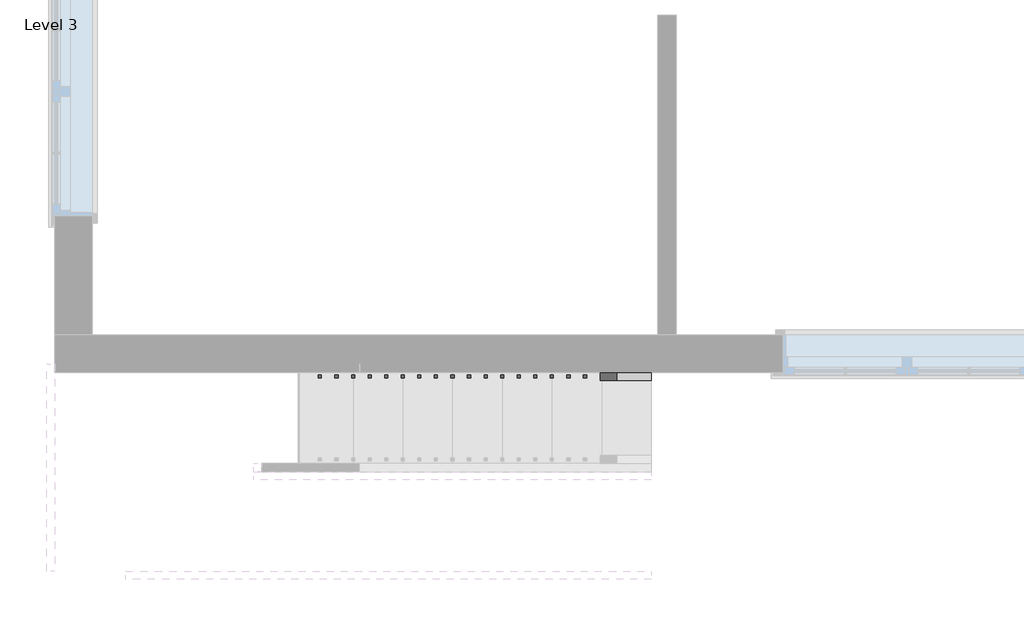
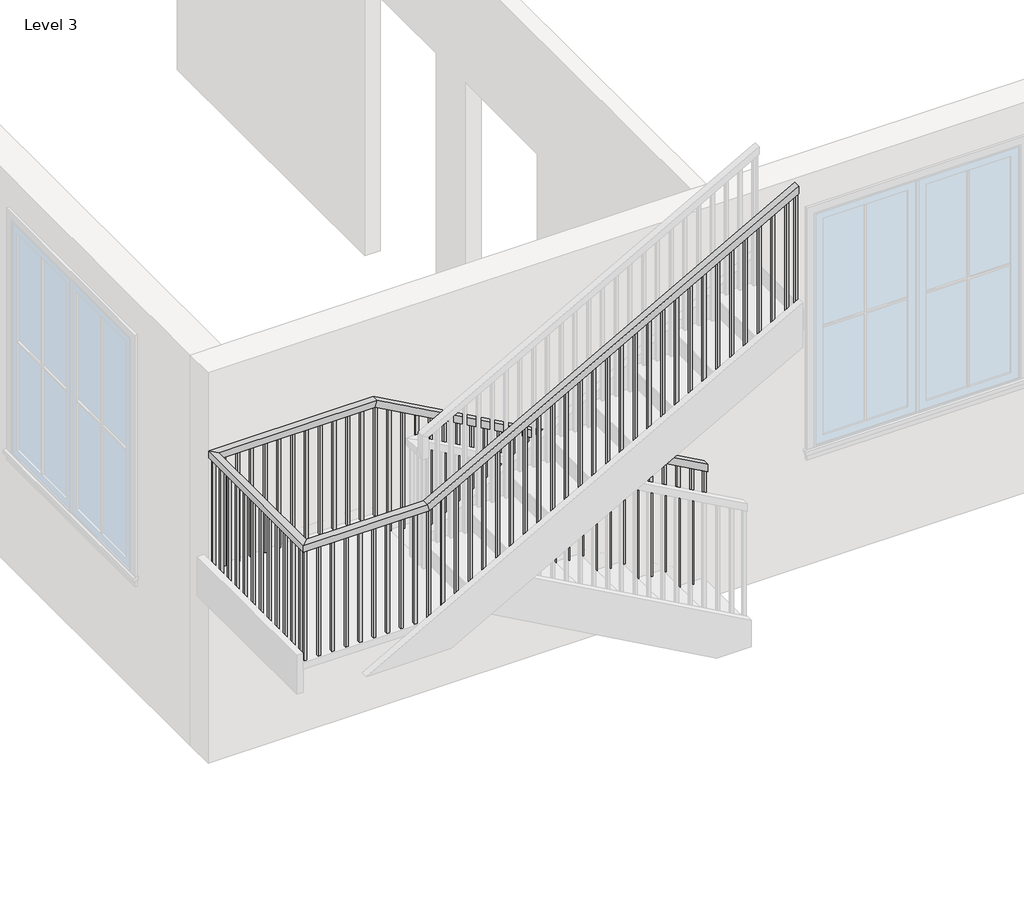
# One storey, part 2 of 3: 1 railing.
"""IFC4 building model written with IfcOpenShell, lengths in millimetres."""

from ifc_helpers import new_model, si_unit, frame, origin, place, context, project, spatial, polyline, outline, extrude, faceted_brep, element, save

model = new_model("IFC4")

# Units and contexts
model_context = context("Model", 3, world=origin())
ifc_project = project(units=[si_unit("LENGTHUNIT", "METRE", prefix="MILLI")], contexts=[model_context])

# Site, building, storey
site = spatial("IfcSite", under=ifc_project)
building = spatial("IfcBuilding", under=site)
storey = spatial("IfcBuildingStorey", under=building, Name="Level 3", Elevation=3200.4)

# Railing
placement = place(None, origin())
element("IfcRailing", 1, ObjectType="Handrail - Rectangular", at=placement, inside=storey, context=model_context, shape_type="SolidModel", body=[
    faceted_brep([(-1805.9198569, -5357.1933037, 4284.1333333), (-1805.9198569, -5357.1933037, 4226.020221), (-1805.9198569, -5306.3933037, 4226.020221), (-1805.9198569, -5306.3933037, 4284.1333333), (-4244.3198569, -5357.1933037, 5638.8), (-4257.4834592, -5357.1933037, 5588.0), (-4257.4834592, -5306.3933037, 5588.0), (-4244.3198569, -5306.3933037, 5638.8), (-5412.7198569, -5357.1933037, 5638.8), (-5412.7198569, -5357.1933037, 5588.0), (-5463.5198569, -5306.3933037, 5588.0), (-5463.5198569, -5306.3933037, 5638.8), (-5412.7198569, -6474.7933037, 5638.8), (-5412.7198569, -6474.7933037, 5588.0), (-5463.5198569, -6525.5933037, 5588.0), (-5463.5198569, -6525.5933037, 5638.8), (-4549.1198569, -6474.7933037, 5638.8), (-4535.9562547, -6474.7933037, 5588.0), (-4535.9562547, -6525.5933037, 5588.0), (-4549.1198569, -6525.5933037, 5638.8), (-1805.9198569, -6474.7933037, 7162.8), (-1805.9198569, -6525.5933037, 7162.8), (-1805.9198569, -6525.5933037, 7104.6868876), (-1805.9198569, -6474.7933037, 7104.6868876)], [[[0, 1, 2, 3]], [[1, 0, 4, 5]], [[2, 1, 5, 6]], [[3, 2, 6, 7]], [[0, 3, 7, 4]], [[5, 4, 8, 9]], [[6, 5, 9, 10]], [[7, 6, 10, 11]], [[4, 7, 11, 8]], [[9, 8, 12, 13]], [[10, 9, 13, 14]], [[11, 10, 14, 15]], [[8, 11, 15, 12]], [[13, 12, 16, 17]], [[14, 13, 17, 18]], [[15, 14, 18, 19]], [[12, 15, 19, 16]], [[20, 21, 22, 23]], [[17, 16, 20, 23]], [[18, 17, 23, 22]], [[19, 18, 22, 21]], [[16, 19, 21, 20]]]),
    extrude(outline(polyline([(7067.645221, -1872.5948569), (7057.0618876, -1891.6448569), (6079.0666667, -1891.6448569), (6079.0666667, -1872.5948569), (7067.645221, -1872.5948569)])), frame((0.0, -6509.7183037, 0.0), z_axis=(0.0, 1.0, 0.0), x_axis=(0.0, 0.0, 1.0)), (0.0, 0.0, 1.0), 19.05),
    extrude(outline(polyline([(7011.2007765, -1974.1948569), (7000.6174432, -1993.2448569), (6079.0666667, -1993.2448569), (6079.0666667, -1974.1948569), (7011.2007765, -1974.1948569)])), frame((0.0, -6509.7183037, 0.0), z_axis=(0.0, 1.0, 0.0), x_axis=(0.0, 0.0, 1.0)), (0.0, 0.0, 1.0), 19.05),
    extrude(outline(polyline([(6954.7563321, -2075.7948569), (6944.1729988, -2094.8448569), (6079.0666667, -2094.8448569), (6079.0666667, -2075.7948569), (6954.7563321, -2075.7948569)])), frame((0.0, -6509.7183037, 0.0), z_axis=(0.0, 1.0, 0.0), x_axis=(0.0, 0.0, 1.0)), (0.0, 0.0, 1.0), 19.05),
    extrude(outline(polyline([(6898.3118876, -2177.3948569), (6887.7285543, -2196.4448569), (5909.7333333, -2196.4448569), (5909.7333333, -2177.3948569), (6898.3118876, -2177.3948569)])), frame((0.0, -6509.7183037, 0.0), z_axis=(0.0, 1.0, 0.0), x_axis=(0.0, 0.0, 1.0)), (0.0, 0.0, 1.0), 19.05),
    extrude(outline(polyline([(6841.8674432, -2278.9948569), (6831.2841099, -2298.0448569), (5909.7333333, -2298.0448569), (5909.7333333, -2278.9948569), (6841.8674432, -2278.9948569)])), frame((0.0, -6509.7183037, 0.0), z_axis=(0.0, 1.0, 0.0), x_axis=(0.0, 0.0, 1.0)), (0.0, 0.0, 1.0), 19.05),
    extrude(outline(polyline([(6785.4229988, -2380.5948569), (6774.8396654, -2399.6448569), (5909.7333333, -2399.6448569), (5909.7333333, -2380.5948569), (6785.4229988, -2380.5948569)])), frame((0.0, -6509.7183037, 0.0), z_axis=(0.0, 1.0, 0.0), x_axis=(0.0, 0.0, 1.0)), (0.0, 0.0, 1.0), 19.05),
    extrude(outline(polyline([(6728.9785543, -2482.1948569), (6718.395221, -2501.2448569), (5740.4, -2501.2448569), (5740.4, -2482.1948569), (6728.9785543, -2482.1948569)])), frame((0.0, -6509.7183037, 0.0), z_axis=(0.0, 1.0, 0.0), x_axis=(0.0, 0.0, 1.0)), (0.0, 0.0, 1.0), 19.05),
    extrude(outline(polyline([(6672.5341099, -2583.7948569), (6661.9507765, -2602.8448569), (5740.4, -2602.8448569), (5740.4, -2583.7948569), (6672.5341099, -2583.7948569)])), frame((0.0, -6509.7183037, 0.0), z_axis=(0.0, 1.0, 0.0), x_axis=(0.0, 0.0, 1.0)), (0.0, 0.0, 1.0), 19.05),
    extrude(outline(polyline([(6616.0896654, -2685.3948569), (6605.5063321, -2704.4448569), (5740.4, -2704.4448569), (5740.4, -2685.3948569), (6616.0896654, -2685.3948569)])), frame((0.0, -6509.7183037, 0.0), z_axis=(0.0, 1.0, 0.0), x_axis=(0.0, 0.0, 1.0)), (0.0, 0.0, 1.0), 19.05),
    extrude(outline(polyline([(6559.645221, -2786.9948569), (6549.0618876, -2806.0448569), (5571.0666667, -2806.0448569), (5571.0666667, -2786.9948569), (6559.645221, -2786.9948569)])), frame((0.0, -6509.7183037, 0.0), z_axis=(0.0, 1.0, 0.0), x_axis=(0.0, 0.0, 1.0)), (0.0, 0.0, 1.0), 19.05),
    extrude(outline(polyline([(6503.2007765, -2888.5948569), (6492.6174432, -2907.6448569), (5571.0666667, -2907.6448569), (5571.0666667, -2888.5948569), (6503.2007765, -2888.5948569)])), frame((0.0, -6509.7183037, 0.0), z_axis=(0.0, 1.0, 0.0), x_axis=(0.0, 0.0, 1.0)), (0.0, 0.0, 1.0), 19.05),
    extrude(outline(polyline([(6446.7563321, -2990.1948569), (6436.1729988, -3009.2448569), (5571.0666667, -3009.2448569), (5571.0666667, -2990.1948569), (6446.7563321, -2990.1948569)])), frame((0.0, -6509.7183037, 0.0), z_axis=(0.0, 1.0, 0.0), x_axis=(0.0, 0.0, 1.0)), (0.0, 0.0, 1.0), 19.05),
    extrude(outline(polyline([(6390.3118876, -3091.7948569), (6379.7285543, -3110.8448569), (5401.7333333, -3110.8448569), (5401.7333333, -3091.7948569), (6390.3118876, -3091.7948569)])), frame((0.0, -6509.7183037, 0.0), z_axis=(0.0, 1.0, 0.0), x_axis=(0.0, 0.0, 1.0)), (0.0, 0.0, 1.0), 19.05),
    extrude(outline(polyline([(6333.8674432, -3193.3948569), (6323.2841099, -3212.4448569), (5401.7333333, -3212.4448569), (5401.7333333, -3193.3948569), (6333.8674432, -3193.3948569)])), frame((0.0, -6509.7183037, 0.0), z_axis=(0.0, 1.0, 0.0), x_axis=(0.0, 0.0, 1.0)), (0.0, 0.0, 1.0), 19.05),
    extrude(outline(polyline([(6277.4229988, -3294.9948569), (6266.8396654, -3314.0448569), (5401.7333333, -3314.0448569), (5401.7333333, -3294.9948569), (6277.4229988, -3294.9948569)])), frame((0.0, -6509.7183037, 0.0), z_axis=(0.0, 1.0, 0.0), x_axis=(0.0, 0.0, 1.0)), (0.0, 0.0, 1.0), 19.05),
    extrude(outline(polyline([(6220.9785543, -3396.5948569), (6210.395221, -3415.6448569), (5232.4, -3415.6448569), (5232.4, -3396.5948569), (6220.9785543, -3396.5948569)])), frame((0.0, -6509.7183037, 0.0), z_axis=(0.0, 1.0, 0.0), x_axis=(0.0, 0.0, 1.0)), (0.0, 0.0, 1.0), 19.05),
    extrude(outline(polyline([(6164.5341099, -3498.1948569), (6153.9507765, -3517.2448569), (5232.4, -3517.2448569), (5232.4, -3498.1948569), (6164.5341099, -3498.1948569)])), frame((0.0, -6509.7183037, 0.0), z_axis=(0.0, 1.0, 0.0), x_axis=(0.0, 0.0, 1.0)), (0.0, 0.0, 1.0), 19.05),
    extrude(outline(polyline([(6108.0896654, -3599.7948569), (6097.5063321, -3618.8448569), (5232.4, -3618.8448569), (5232.4, -3599.7948569), (6108.0896654, -3599.7948569)])), frame((0.0, -6509.7183037, 0.0), z_axis=(0.0, 1.0, 0.0), x_axis=(0.0, 0.0, 1.0)), (0.0, 0.0, 1.0), 19.05),
    extrude(outline(polyline([(6051.645221, -3701.3948569), (6041.0618876, -3720.4448569), (5063.0666667, -3720.4448569), (5063.0666667, -3701.3948569), (6051.645221, -3701.3948569)])), frame((0.0, -6509.7183037, 0.0), z_axis=(0.0, 1.0, 0.0), x_axis=(0.0, 0.0, 1.0)), (0.0, 0.0, 1.0), 19.05),
    extrude(outline(polyline([(5995.2007765, -3802.9948569), (5984.6174432, -3822.0448569), (5063.0666667, -3822.0448569), (5063.0666667, -3802.9948569), (5995.2007765, -3802.9948569)])), frame((0.0, -6509.7183037, 0.0), z_axis=(0.0, 1.0, 0.0), x_axis=(0.0, 0.0, 1.0)), (0.0, 0.0, 1.0), 19.05),
    extrude(outline(polyline([(5938.7563321, -3904.5948569), (5928.1729988, -3923.6448569), (5063.0666667, -3923.6448569), (5063.0666667, -3904.5948569), (5938.7563321, -3904.5948569)])), frame((0.0, -6509.7183037, 0.0), z_axis=(0.0, 1.0, 0.0), x_axis=(0.0, 0.0, 1.0)), (0.0, 0.0, 1.0), 19.05),
    extrude(outline(polyline([(5882.3118876, -4006.1948569), (5871.7285543, -4025.2448569), (4893.7333333, -4025.2448569), (4893.7333333, -4006.1948569), (5882.3118876, -4006.1948569)])), frame((0.0, -6509.7183037, 0.0), z_axis=(0.0, 1.0, 0.0), x_axis=(0.0, 0.0, 1.0)), (0.0, 0.0, 1.0), 19.05),
    extrude(outline(polyline([(5825.8674432, -4107.7948569), (5815.2841099, -4126.8448569), (4893.7333333, -4126.8448569), (4893.7333333, -4107.7948569), (5825.8674432, -4107.7948569)])), frame((0.0, -6509.7183037, 0.0), z_axis=(0.0, 1.0, 0.0), x_axis=(0.0, 0.0, 1.0)), (0.0, 0.0, 1.0), 19.05),
    extrude(outline(polyline([(5769.4229988, -4209.3948569), (5758.8396654, -4228.4448569), (4893.7333333, -4228.4448569), (4893.7333333, -4209.3948569), (5769.4229988, -4209.3948569)])), frame((0.0, -6509.7183037, 0.0), z_axis=(0.0, 1.0, 0.0), x_axis=(0.0, 0.0, 1.0)), (0.0, 0.0, 1.0), 19.05),
    extrude(outline(polyline([(5712.9785543, -4310.9948569), (5702.395221, -4330.0448569), (4724.4, -4330.0448569), (4724.4, -4310.9948569), (5712.9785543, -4310.9948569)])), frame((0.0, -6509.7183037, 0.0), z_axis=(0.0, 1.0, 0.0), x_axis=(0.0, 0.0, 1.0)), (0.0, 0.0, 1.0), 19.05),
    extrude(outline(polyline([(5656.5341099, -4412.5948569), (5645.9507765, -4431.6448569), (4724.4, -4431.6448569), (4724.4, -4412.5948569), (5656.5341099, -4412.5948569)])), frame((0.0, -6509.7183037, 0.0), z_axis=(0.0, 1.0, 0.0), x_axis=(0.0, 0.0, 1.0)), (0.0, 0.0, 1.0), 19.05),
    extrude(outline(polyline([(5600.0896654, -4514.1948569), (5589.5063321, -4533.2448569), (4724.4, -4533.2448569), (4724.4, -4514.1948569), (5600.0896654, -4514.1948569)])), frame((0.0, -6509.7183037, 0.0), z_axis=(0.0, 1.0, 0.0), x_axis=(0.0, 0.0, 1.0)), (0.0, 0.0, 1.0), 19.05),
    extrude(outline(polyline([(-4634.8448569, -6509.7183037), (-4634.8448569, -6490.6683037), (-4615.7948569, -6490.6683037), (-4615.7948569, -6509.7183037), (-4634.8448569, -6509.7183037)])), frame((0.0, 0.0, 4724.4), z_axis=(0.0, 0.0, 1.0), x_axis=(1.0, 0.0, 0.0)), (0.0, 0.0, 1.0), 863.6),
    extrude(outline(polyline([(-4736.4448569, -6509.7183037), (-4736.4448569, -6490.6683037), (-4717.3948569, -6490.6683037), (-4717.3948569, -6509.7183037), (-4736.4448569, -6509.7183037)])), frame((0.0, 0.0, 4724.4), z_axis=(0.0, 0.0, 1.0), x_axis=(1.0, 0.0, 0.0)), (0.0, 0.0, 1.0), 863.6),
    extrude(outline(polyline([(-4838.0448569, -6509.7183037), (-4838.0448569, -6490.6683037), (-4818.9948569, -6490.6683037), (-4818.9948569, -6509.7183037), (-4838.0448569, -6509.7183037)])), frame((0.0, 0.0, 4724.4), z_axis=(0.0, 0.0, 1.0), x_axis=(1.0, 0.0, 0.0)), (0.0, 0.0, 1.0), 863.6),
    extrude(outline(polyline([(-4939.6448569, -6509.7183037), (-4939.6448569, -6490.6683037), (-4920.5948569, -6490.6683037), (-4920.5948569, -6509.7183037), (-4939.6448569, -6509.7183037)])), frame((0.0, 0.0, 4724.4), z_axis=(0.0, 0.0, 1.0), x_axis=(1.0, 0.0, 0.0)), (0.0, 0.0, 1.0), 863.6),
    extrude(outline(polyline([(-5041.2448569, -6509.7183037), (-5041.2448569, -6490.6683037), (-5022.1948569, -6490.6683037), (-5022.1948569, -6509.7183037), (-5041.2448569, -6509.7183037)])), frame((0.0, 0.0, 4724.4), z_axis=(0.0, 0.0, 1.0), x_axis=(1.0, 0.0, 0.0)), (0.0, 0.0, 1.0), 863.6),
    extrude(outline(polyline([(-5142.8448569, -6509.7183037), (-5142.8448569, -6490.6683037), (-5123.7948569, -6490.6683037), (-5123.7948569, -6509.7183037), (-5142.8448569, -6509.7183037)])), frame((0.0, 0.0, 4724.4), z_axis=(0.0, 0.0, 1.0), x_axis=(1.0, 0.0, 0.0)), (0.0, 0.0, 1.0), 863.6),
    extrude(outline(polyline([(-5244.4448569, -6509.7183037), (-5244.4448569, -6490.6683037), (-5225.3948569, -6490.6683037), (-5225.3948569, -6509.7183037), (-5244.4448569, -6509.7183037)])), frame((0.0, 0.0, 4724.4), z_axis=(0.0, 0.0, 1.0), x_axis=(1.0, 0.0, 0.0)), (0.0, 0.0, 1.0), 863.6),
    extrude(outline(polyline([(-5346.0448569, -6509.7183037), (-5346.0448569, -6490.6683037), (-5326.9948569, -6490.6683037), (-5326.9948569, -6509.7183037), (-5346.0448569, -6509.7183037)])), frame((0.0, 0.0, 4724.4), z_axis=(0.0, 0.0, 1.0), x_axis=(1.0, 0.0, 0.0)), (0.0, 0.0, 1.0), 863.6),
    extrude(outline(polyline([(-5447.6448569, -6439.8683037), (-5428.5948569, -6439.8683037), (-5428.5948569, -6458.9183037), (-5447.6448569, -6458.9183037), (-5447.6448569, -6439.8683037)])), frame((0.0, 0.0, 4724.4), z_axis=(0.0, 0.0, 1.0), x_axis=(1.0, 0.0, 0.0)), (0.0, 0.0, 1.0), 863.6),
    extrude(outline(polyline([(-5447.6448569, -6338.2683037), (-5428.5948569, -6338.2683037), (-5428.5948569, -6357.3183037), (-5447.6448569, -6357.3183037), (-5447.6448569, -6338.2683037)])), frame((0.0, 0.0, 4724.4), z_axis=(0.0, 0.0, 1.0), x_axis=(1.0, 0.0, 0.0)), (0.0, 0.0, 1.0), 863.6),
    extrude(outline(polyline([(-5447.6448569, -6236.6683037), (-5428.5948569, -6236.6683037), (-5428.5948569, -6255.7183037), (-5447.6448569, -6255.7183037), (-5447.6448569, -6236.6683037)])), frame((0.0, 0.0, 4724.4), z_axis=(0.0, 0.0, 1.0), x_axis=(1.0, 0.0, 0.0)), (0.0, 0.0, 1.0), 863.6),
    extrude(outline(polyline([(-5447.6448569, -6135.0683037), (-5428.5948569, -6135.0683037), (-5428.5948569, -6154.1183037), (-5447.6448569, -6154.1183037), (-5447.6448569, -6135.0683037)])), frame((0.0, 0.0, 4724.4), z_axis=(0.0, 0.0, 1.0), x_axis=(1.0, 0.0, 0.0)), (0.0, 0.0, 1.0), 863.6),
    extrude(outline(polyline([(-5447.6448569, -6033.4683037), (-5428.5948569, -6033.4683037), (-5428.5948569, -6052.5183037), (-5447.6448569, -6052.5183037), (-5447.6448569, -6033.4683037)])), frame((0.0, 0.0, 4724.4), z_axis=(0.0, 0.0, 1.0), x_axis=(1.0, 0.0, 0.0)), (0.0, 0.0, 1.0), 863.6),
    extrude(outline(polyline([(-5447.6448569, -5931.8683037), (-5428.5948569, -5931.8683037), (-5428.5948569, -5950.9183037), (-5447.6448569, -5950.9183037), (-5447.6448569, -5931.8683037)])), frame((0.0, 0.0, 4724.4), z_axis=(0.0, 0.0, 1.0), x_axis=(1.0, 0.0, 0.0)), (0.0, 0.0, 1.0), 863.6),
    extrude(outline(polyline([(-5447.6448569, -5830.2683037), (-5428.5948569, -5830.2683037), (-5428.5948569, -5849.3183037), (-5447.6448569, -5849.3183037), (-5447.6448569, -5830.2683037)])), frame((0.0, 0.0, 4724.4), z_axis=(0.0, 0.0, 1.0), x_axis=(1.0, 0.0, 0.0)), (0.0, 0.0, 1.0), 863.6),
    extrude(outline(polyline([(-5447.6448569, -5728.6683037), (-5428.5948569, -5728.6683037), (-5428.5948569, -5747.7183037), (-5447.6448569, -5747.7183037), (-5447.6448569, -5728.6683037)])), frame((0.0, 0.0, 4724.4), z_axis=(0.0, 0.0, 1.0), x_axis=(1.0, 0.0, 0.0)), (0.0, 0.0, 1.0), 863.6),
    extrude(outline(polyline([(-5447.6448569, -5627.0683037), (-5428.5948569, -5627.0683037), (-5428.5948569, -5646.1183037), (-5447.6448569, -5646.1183037), (-5447.6448569, -5627.0683037)])), frame((0.0, 0.0, 4724.4), z_axis=(0.0, 0.0, 1.0), x_axis=(1.0, 0.0, 0.0)), (0.0, 0.0, 1.0), 863.6),
    extrude(outline(polyline([(-5447.6448569, -5525.4683037), (-5428.5948569, -5525.4683037), (-5428.5948569, -5544.5183037), (-5447.6448569, -5544.5183037), (-5447.6448569, -5525.4683037)])), frame((0.0, 0.0, 4724.4), z_axis=(0.0, 0.0, 1.0), x_axis=(1.0, 0.0, 0.0)), (0.0, 0.0, 1.0), 863.6),
    extrude(outline(polyline([(-5447.6448569, -5423.8683037), (-5428.5948569, -5423.8683037), (-5428.5948569, -5442.9183037), (-5447.6448569, -5442.9183037), (-5447.6448569, -5423.8683037)])), frame((0.0, 0.0, 4724.4), z_axis=(0.0, 0.0, 1.0), x_axis=(1.0, 0.0, 0.0)), (0.0, 0.0, 1.0), 863.6),
    extrude(outline(polyline([(-5352.3948569, -5322.2683037), (-5352.3948569, -5341.3183037), (-5371.4448569, -5341.3183037), (-5371.4448569, -5322.2683037), (-5352.3948569, -5322.2683037)])), frame((0.0, 0.0, 4724.4), z_axis=(0.0, 0.0, 1.0), x_axis=(1.0, 0.0, 0.0)), (0.0, 0.0, 1.0), 863.6),
    extrude(outline(polyline([(-5250.7948569, -5322.2683037), (-5250.7948569, -5341.3183037), (-5269.8448569, -5341.3183037), (-5269.8448569, -5322.2683037), (-5250.7948569, -5322.2683037)])), frame((0.0, 0.0, 4724.4), z_axis=(0.0, 0.0, 1.0), x_axis=(1.0, 0.0, 0.0)), (0.0, 0.0, 1.0), 863.6),
    extrude(outline(polyline([(-5149.1948569, -5322.2683037), (-5149.1948569, -5341.3183037), (-5168.2448569, -5341.3183037), (-5168.2448569, -5322.2683037), (-5149.1948569, -5322.2683037)])), frame((0.0, 0.0, 4724.4), z_axis=(0.0, 0.0, 1.0), x_axis=(1.0, 0.0, 0.0)), (0.0, 0.0, 1.0), 863.6),
    extrude(outline(polyline([(-5047.5948569, -5322.2683037), (-5047.5948569, -5341.3183037), (-5066.6448569, -5341.3183037), (-5066.6448569, -5322.2683037), (-5047.5948569, -5322.2683037)])), frame((0.0, 0.0, 4724.4), z_axis=(0.0, 0.0, 1.0), x_axis=(1.0, 0.0, 0.0)), (0.0, 0.0, 1.0), 863.6),
    extrude(outline(polyline([(-4945.9948569, -5322.2683037), (-4945.9948569, -5341.3183037), (-4965.0448569, -5341.3183037), (-4965.0448569, -5322.2683037), (-4945.9948569, -5322.2683037)])), frame((0.0, 0.0, 4724.4), z_axis=(0.0, 0.0, 1.0), x_axis=(1.0, 0.0, 0.0)), (0.0, 0.0, 1.0), 863.6),
    extrude(outline(polyline([(-4844.3948569, -5322.2683037), (-4844.3948569, -5341.3183037), (-4863.4448569, -5341.3183037), (-4863.4448569, -5322.2683037), (-4844.3948569, -5322.2683037)])), frame((0.0, 0.0, 4724.4), z_axis=(0.0, 0.0, 1.0), x_axis=(1.0, 0.0, 0.0)), (0.0, 0.0, 1.0), 863.6),
    extrude(outline(polyline([(-4742.7948569, -5322.2683037), (-4742.7948569, -5341.3183037), (-4761.8448569, -5341.3183037), (-4761.8448569, -5322.2683037), (-4742.7948569, -5322.2683037)])), frame((0.0, 0.0, 4724.4), z_axis=(0.0, 0.0, 1.0), x_axis=(1.0, 0.0, 0.0)), (0.0, 0.0, 1.0), 863.6),
    extrude(outline(polyline([(-4641.1948569, -5322.2683037), (-4641.1948569, -5341.3183037), (-4660.2448569, -5341.3183037), (-4660.2448569, -5322.2683037), (-4641.1948569, -5322.2683037)])), frame((0.0, 0.0, 4724.4), z_axis=(0.0, 0.0, 1.0), x_axis=(1.0, 0.0, 0.0)), (0.0, 0.0, 1.0), 863.6),
    extrude(outline(polyline([(-4539.5948569, -5322.2683037), (-4539.5948569, -5341.3183037), (-4558.6448569, -5341.3183037), (-4558.6448569, -5322.2683037), (-4539.5948569, -5322.2683037)])), frame((0.0, 0.0, 4724.4), z_axis=(0.0, 0.0, 1.0), x_axis=(1.0, 0.0, 0.0)), (0.0, 0.0, 1.0), 863.6),
    extrude(outline(polyline([(-4437.9948569, -5322.2683037), (-4437.9948569, -5341.3183037), (-4457.0448569, -5341.3183037), (-4457.0448569, -5322.2683037), (-4437.9948569, -5322.2683037)])), frame((0.0, 0.0, 4724.4), z_axis=(0.0, 0.0, 1.0), x_axis=(1.0, 0.0, 0.0)), (0.0, 0.0, 1.0), 863.6),
    extrude(outline(polyline([(-4336.3948569, -5322.2683037), (-4336.3948569, -5341.3183037), (-4355.4448569, -5341.3183037), (-4355.4448569, -5322.2683037), (-4336.3948569, -5322.2683037)])), frame((0.0, 0.0, 4724.4), z_axis=(0.0, 0.0, 1.0), x_axis=(1.0, 0.0, 0.0)), (0.0, 0.0, 1.0), 863.6),
    extrude(outline(polyline([(5575.395221, -4234.7948569), (5585.9785543, -4253.8448569), (4724.4, -4253.8448569), (4724.4, -4234.7948569), (5575.395221, -4234.7948569)])), frame((0.0, -5341.3183037, 0.0), z_axis=(0.0, 1.0, 0.0), x_axis=(0.0, 0.0, 1.0)), (0.0, 0.0, 1.0), 19.05),
    extrude(outline(polyline([(5518.9507765, -4133.1948569), (5529.5341099, -4152.2448569), (4555.0666667, -4152.2448569), (4555.0666667, -4133.1948569), (5518.9507765, -4133.1948569)])), frame((0.0, -5341.3183037, 0.0), z_axis=(0.0, 1.0, 0.0), x_axis=(0.0, 0.0, 1.0)), (0.0, 0.0, 1.0), 19.05),
    extrude(outline(polyline([(5462.5063321, -4031.5948569), (5473.0896654, -4050.6448569), (4555.0666667, -4050.6448569), (4555.0666667, -4031.5948569), (5462.5063321, -4031.5948569)])), frame((0.0, -5341.3183037, 0.0), z_axis=(0.0, 1.0, 0.0), x_axis=(0.0, 0.0, 1.0)), (0.0, 0.0, 1.0), 19.05),
    extrude(outline(polyline([(5406.0618876, -3929.9948569), (5416.645221, -3949.0448569), (4555.0666667, -3949.0448569), (4555.0666667, -3929.9948569), (5406.0618876, -3929.9948569)])), frame((0.0, -5341.3183037, 0.0), z_axis=(0.0, 1.0, 0.0), x_axis=(0.0, 0.0, 1.0)), (0.0, 0.0, 1.0), 19.05),
    extrude(outline(polyline([(5349.6174432, -3828.3948569), (5360.2007765, -3847.4448569), (4385.7333333, -3847.4448569), (4385.7333333, -3828.3948569), (5349.6174432, -3828.3948569)])), frame((0.0, -5341.3183037, 0.0), z_axis=(0.0, 1.0, 0.0), x_axis=(0.0, 0.0, 1.0)), (0.0, 0.0, 1.0), 19.05),
    extrude(outline(polyline([(5293.1729988, -3726.7948569), (5303.7563321, -3745.8448569), (4385.7333333, -3745.8448569), (4385.7333333, -3726.7948569), (5293.1729988, -3726.7948569)])), frame((0.0, -5341.3183037, 0.0), z_axis=(0.0, 1.0, 0.0), x_axis=(0.0, 0.0, 1.0)), (0.0, 0.0, 1.0), 19.05),
    extrude(outline(polyline([(5236.7285543, -3625.1948569), (5247.3118876, -3644.2448569), (4385.7333333, -3644.2448569), (4385.7333333, -3625.1948569), (5236.7285543, -3625.1948569)])), frame((0.0, -5341.3183037, 0.0), z_axis=(0.0, 1.0, 0.0), x_axis=(0.0, 0.0, 1.0)), (0.0, 0.0, 1.0), 19.05),
    extrude(outline(polyline([(5180.2841099, -3523.5948569), (5190.8674432, -3542.6448569), (4216.4, -3542.6448569), (4216.4, -3523.5948569), (5180.2841099, -3523.5948569)])), frame((0.0, -5341.3183037, 0.0), z_axis=(0.0, 1.0, 0.0), x_axis=(0.0, 0.0, 1.0)), (0.0, 0.0, 1.0), 19.05),
    extrude(outline(polyline([(5123.8396654, -3421.9948569), (5134.4229988, -3441.0448569), (4216.4, -3441.0448569), (4216.4, -3421.9948569), (5123.8396654, -3421.9948569)])), frame((0.0, -5341.3183037, 0.0), z_axis=(0.0, 1.0, 0.0), x_axis=(0.0, 0.0, 1.0)), (0.0, 0.0, 1.0), 19.05),
    extrude(outline(polyline([(5067.395221, -3320.3948569), (5077.9785543, -3339.4448569), (4216.4, -3339.4448569), (4216.4, -3320.3948569), (5067.395221, -3320.3948569)])), frame((0.0, -5341.3183037, 0.0), z_axis=(0.0, 1.0, 0.0), x_axis=(0.0, 0.0, 1.0)), (0.0, 0.0, 1.0), 19.05),
    extrude(outline(polyline([(5010.9507765, -3218.7948569), (5021.5341099, -3237.8448569), (4047.0666667, -3237.8448569), (4047.0666667, -3218.7948569), (5010.9507765, -3218.7948569)])), frame((0.0, -5341.3183037, 0.0), z_axis=(0.0, 1.0, 0.0), x_axis=(0.0, 0.0, 1.0)), (0.0, 0.0, 1.0), 19.05),
    extrude(outline(polyline([(4954.5063321, -3117.1948569), (4965.0896654, -3136.2448569), (4047.0666667, -3136.2448569), (4047.0666667, -3117.1948569), (4954.5063321, -3117.1948569)])), frame((0.0, -5341.3183037, 0.0), z_axis=(0.0, 1.0, 0.0), x_axis=(0.0, 0.0, 1.0)), (0.0, 0.0, 1.0), 19.05),
    extrude(outline(polyline([(4898.0618876, -3015.5948569), (4908.645221, -3034.6448569), (4047.0666667, -3034.6448569), (4047.0666667, -3015.5948569), (4898.0618876, -3015.5948569)])), frame((0.0, -5341.3183037, 0.0), z_axis=(0.0, 1.0, 0.0), x_axis=(0.0, 0.0, 1.0)), (0.0, 0.0, 1.0), 19.05),
    extrude(outline(polyline([(4841.6174432, -2913.9948569), (4852.2007765, -2933.0448569), (3877.7333333, -2933.0448569), (3877.7333333, -2913.9948569), (4841.6174432, -2913.9948569)])), frame((0.0, -5341.3183037, 0.0), z_axis=(0.0, 1.0, 0.0), x_axis=(0.0, 0.0, 1.0)), (0.0, 0.0, 1.0), 19.05),
    extrude(outline(polyline([(4785.1729988, -2812.3948569), (4795.7563321, -2831.4448569), (3877.7333333, -2831.4448569), (3877.7333333, -2812.3948569), (4785.1729988, -2812.3948569)])), frame((0.0, -5341.3183037, 0.0), z_axis=(0.0, 1.0, 0.0), x_axis=(0.0, 0.0, 1.0)), (0.0, 0.0, 1.0), 19.05),
    extrude(outline(polyline([(4728.7285543, -2710.7948569), (4739.3118876, -2729.8448569), (3877.7333333, -2729.8448569), (3877.7333333, -2710.7948569), (4728.7285543, -2710.7948569)])), frame((0.0, -5341.3183037, 0.0), z_axis=(0.0, 1.0, 0.0), x_axis=(0.0, 0.0, 1.0)), (0.0, 0.0, 1.0), 19.05),
    extrude(outline(polyline([(4672.2841099, -2609.1948569), (4682.8674432, -2628.2448569), (3708.4, -2628.2448569), (3708.4, -2609.1948569), (4672.2841099, -2609.1948569)])), frame((0.0, -5341.3183037, 0.0), z_axis=(0.0, 1.0, 0.0), x_axis=(0.0, 0.0, 1.0)), (0.0, 0.0, 1.0), 19.05),
    extrude(outline(polyline([(4615.8396654, -2507.5948569), (4626.4229988, -2526.6448569), (3708.4, -2526.6448569), (3708.4, -2507.5948569), (4615.8396654, -2507.5948569)])), frame((0.0, -5341.3183037, 0.0), z_axis=(0.0, 1.0, 0.0), x_axis=(0.0, 0.0, 1.0)), (0.0, 0.0, 1.0), 19.05),
    extrude(outline(polyline([(4559.395221, -2405.9948569), (4569.9785543, -2425.0448569), (3708.4, -2425.0448569), (3708.4, -2405.9948569), (4559.395221, -2405.9948569)])), frame((0.0, -5341.3183037, 0.0), z_axis=(0.0, 1.0, 0.0), x_axis=(0.0, 0.0, 1.0)), (0.0, 0.0, 1.0), 19.05),
    extrude(outline(polyline([(4502.9507765, -2304.3948569), (4513.5341099, -2323.4448569), (3539.0666667, -2323.4448569), (3539.0666667, -2304.3948569), (4502.9507765, -2304.3948569)])), frame((0.0, -5341.3183037, 0.0), z_axis=(0.0, 1.0, 0.0), x_axis=(0.0, 0.0, 1.0)), (0.0, 0.0, 1.0), 19.05),
    extrude(outline(polyline([(4446.5063321, -2202.7948569), (4457.0896654, -2221.8448569), (3539.0666667, -2221.8448569), (3539.0666667, -2202.7948569), (4446.5063321, -2202.7948569)])), frame((0.0, -5341.3183037, 0.0), z_axis=(0.0, 1.0, 0.0), x_axis=(0.0, 0.0, 1.0)), (0.0, 0.0, 1.0), 19.05),
    extrude(outline(polyline([(4390.0618876, -2101.1948569), (4400.645221, -2120.2448569), (3539.0666667, -2120.2448569), (3539.0666667, -2101.1948569), (4390.0618876, -2101.1948569)])), frame((0.0, -5341.3183037, 0.0), z_axis=(0.0, 1.0, 0.0), x_axis=(0.0, 0.0, 1.0)), (0.0, 0.0, 1.0), 19.05),
    extrude(outline(polyline([(4333.6174432, -1999.5948569), (4344.2007765, -2018.6448569), (3369.7333333, -2018.6448569), (3369.7333333, -1999.5948569), (4333.6174432, -1999.5948569)])), frame((0.0, -5341.3183037, 0.0), z_axis=(0.0, 1.0, 0.0), x_axis=(0.0, 0.0, 1.0)), (0.0, 0.0, 1.0), 19.05),
    extrude(outline(polyline([(4277.1729988, -1897.9948569), (4287.7563321, -1917.0448569), (3369.7333333, -1917.0448569), (3369.7333333, -1897.9948569), (4277.1729988, -1897.9948569)])), frame((0.0, -5341.3183037, 0.0), z_axis=(0.0, 1.0, 0.0), x_axis=(0.0, 0.0, 1.0)), (0.0, 0.0, 1.0), 19.05),
    extrude(outline(polyline([(-5447.6448569, -6490.6683037), (-5428.5948569, -6490.6683037), (-5428.5948569, -6509.7183037), (-5447.6448569, -6509.7183037), (-5447.6448569, -6490.6683037)])), frame((0.0, 0.0, 4724.4), z_axis=(0.0, 0.0, 1.0), x_axis=(1.0, 0.0, 0.0)), (0.0, 0.0, 1.0), 863.6),
    extrude(outline(polyline([(-5428.5948569, -5322.2683037), (-5428.5948569, -5341.3183037), (-5447.6448569, -5341.3183037), (-5447.6448569, -5322.2683037), (-5428.5948569, -5322.2683037)])), frame((0.0, 0.0, 4724.4), z_axis=(0.0, 0.0, 1.0), x_axis=(1.0, 0.0, 0.0)), (0.0, 0.0, 1.0), 863.6),
    extrude(outline(polyline([(7104.6868876, -1805.9198569), (7094.1035543, -1824.9698569), (6079.0666667, -1824.9698569), (6079.0666667, -1805.9198569), (7104.6868876, -1805.9198569)])), frame((0.0, -6509.7183037, 0.0), z_axis=(0.0, 1.0, 0.0), x_axis=(0.0, 0.0, 1.0)), (0.0, 0.0, 1.0), 19.05),
    extrude(outline(polyline([(4226.020221, -1805.9198569), (4236.6035543, -1824.9698569), (3369.7333333, -1824.9698569), (3369.7333333, -1805.9198569), (4226.020221, -1805.9198569)])), frame((0.0, -5341.3183037, 0.0), z_axis=(0.0, 1.0, 0.0), x_axis=(0.0, 0.0, 1.0)), (0.0, 0.0, 1.0), 19.05),
])

save(model, "model.ifc")

# Revit data of these elements
# Type "Handrail - Rectangular"
#   Assembly Code = "C2010400"
#   built-in parameter 1008612 = 0.0416667 (stored number, unit not read)
#   built-in parameter 1008611 = 0.0416667 (stored number, unit not read)
#   built-in parameter 1008609 = 0.333333 (stored number, unit not read)
#   built-in parameter 1008604 = 0.166667 (stored number, unit not read)
#   built-in parameter 1008603 = 0.166667 (stored number, unit not read)
#   Railing Height = 3' - 0"
#   built-in parameter 1008630 = 2
#   built-in parameter 1008610 = 2
#   built-in parameter 1008618 = Baluster - Square : 3/4"
# Element 1 (IfcRailing, "Handrail - Rectangular")
#   Phase Created = New Construction
